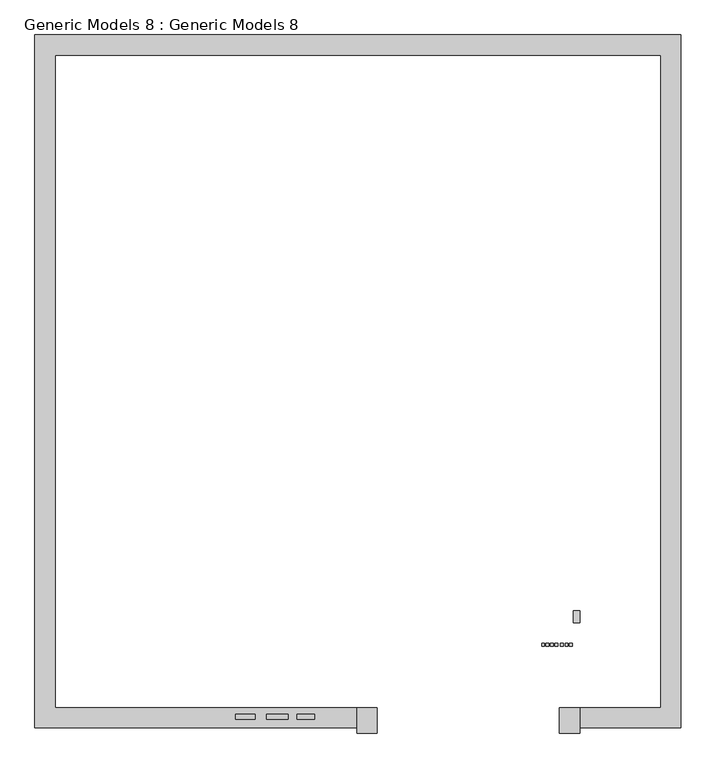
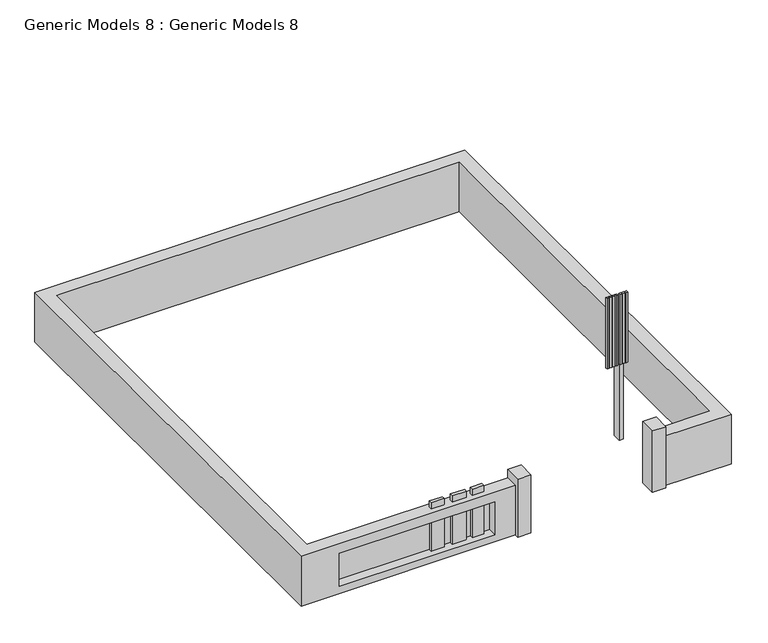
"""IFC4 building model written with IfcOpenShell, lengths in millimetres: proxy geometry, Generic Models 8 : Generic Models 8."""

from ifc_helpers import new_model, si_unit, frame, origin, origin_with_axes, place, context, project, spatial, polyline, outline, extrude, faceted_brep, source, transform, mapped, element, save


def generic_models_8_generic_models_8_408287a0(model_context):
    return source(origin(), model_context, "Body", "SolidModel", [
        extrude(outline(polyline([(-17047.091855, -16063.9538163), (-17567.791855, -16063.9538163), (-17567.791855, -15936.9538163), (-17047.091855, -15936.9538163), (-17047.091855, -16063.9538163)])), origin_with_axes(), (0.0, 0.0, 1.0), 2032.0),
        extrude(outline(polyline([(-16170.791855, -16063.9538163), (-16737.6942581, -16063.9538163), (-16737.6942581, -15936.9538163), (-16170.791855, -15936.9538163), (-16170.791855, -16063.9538163)])), origin_with_axes(), (0.0, 0.0, 1.0), 2032.0),
        extrude(outline(polyline([(-15479.5538452, -16063.9538163), (-15942.191855, -16063.9538163), (-15942.191855, -15936.9538163), (-15479.5538452, -15936.9538163), (-15479.5538452, -16063.9538163)])), origin_with_axes(), (0.0, 0.0, 1.0), 2032.0),
        faceted_brep([(-22861.0806893, -16292.5538163, -304.8), (-22861.0806893, -16292.5538163, 1774.1183755), (-22861.0806893, 1987.5639573, 1774.1183755), (-22861.0806893, 1987.5639573, -304.8), (-22327.6806893, -15759.1538163, -304.8), (-22327.6806893, 1454.1639573, -304.8), (-22327.6806893, 1454.1639573, 1774.1183755), (-22327.6806893, -15759.1538163, 1774.1183755), (-14356.9883599, -15759.1538163, 1774.1183755), (-6340.991855, 1454.1639573, 1774.1183755), (-6340.991855, -15759.1538163, 1774.1183755), (-8474.591855, -15759.1538163, 1774.1183755), (-8474.591855, -16292.5538163, 1774.1183755), (-5807.591855, -16292.5538163, 1774.1183755), (-5807.591855, 1987.5639573, 1774.1183755), (-14356.9883599, -16292.5538163, 1774.1183755), (-14356.9883599, -15759.1538163, -304.8), (-14356.9883599, -16292.5538163, -304.8), (-5807.591855, 1987.5639573, -304.8), (-5807.591855, -16292.5538163, -304.8), (-8474.591855, -16292.5538163, -304.8), (-8474.591855, -15759.1538163, -304.8), (-6340.991855, -15759.1538163, -304.8), (-6340.991855, 1454.1639573, -304.8), (-21339.6745725, -16292.5538163, 0.0), (-21339.6745725, -16292.5538163, 1367.1932574), (-15180.2427002, -16292.5538163, 1367.1932574), (-15180.2427002, -16292.5538163, 0.0), (-21339.6745725, -15936.9538163, 0.0), (-15180.2427002, -15936.9538163, 0.0), (-15180.2427002, -15936.9538163, 1367.1932574), (-21339.6745725, -15936.9538163, 1367.1932574)], [[[0, 1, 2, 3]], [[4, 5, 6, 7]], [[8, 7, 6, 9, 10, 11, 12, 13, 14, 2, 1, 15]], [[4, 16, 17, 0, 3, 18, 19, 20, 21, 22, 23, 5]], [[1, 0, 17, 15], [24, 25, 26, 27]], [[7, 8, 16, 4]], [[15, 17, 16, 8]], [[3, 2, 14, 18]], [[5, 23, 9, 6]], [[14, 13, 19, 18]], [[9, 23, 22, 10]], [[19, 13, 12, 20]], [[22, 21, 11, 10]], [[20, 12, 11, 21]], [[28, 29, 30, 31]], [[28, 31, 25, 24]], [[31, 30, 26, 25]], [[30, 29, 27, 26]], [[29, 28, 24, 27]]]),
        extrude(outline(polyline([(-9007.991855, -16432.2538163), (-9007.991855, -15759.1538163), (-8474.591855, -15759.1538163), (-8474.591855, -16432.2538163), (-9007.991855, -16432.2538163)])), frame((0.0, 0.0, -304.8), z_axis=(0.0, 0.0, 1.0), x_axis=(1.0, 0.0, 0.0)), (0.0, 0.0, 1.0), 2573.6247485),
        extrude(outline(polyline([(-13823.5883599, -15759.1538163), (-13823.5883599, -16432.2538163), (-14356.9883599, -16432.2538163), (-14356.9883599, -15759.1538163), (-13823.5883599, -15759.1538163)])), frame((0.0, 0.0, -304.8), z_axis=(0.0, 0.0, 1.0), x_axis=(1.0, 0.0, 0.0)), (0.0, 0.0, 1.0), 2425.2749439),
        extrude(outline(polyline([(-8745.0065416, -14142.2712123), (-8745.0065416, -14066.0712123), (-8668.8065416, -14066.0712123), (-8668.8065416, -14142.2712123), (-8745.0065416, -14142.2712123)])), frame((0.0, 0.0, 3657.6), z_axis=(0.0, 0.0, 1.0), x_axis=(1.0, 0.0, 0.0)), (0.0, 0.0, 1.0), 2947.4090514),
        extrude(outline(polyline([(-8860.899741, -14142.2712123), (-8860.899741, -14066.0712123), (-8789.0197051, -14066.0712123), (-8789.0197051, -14142.2712123), (-8860.899741, -14142.2712123)])), frame((0.0, 0.0, 3657.6), z_axis=(0.0, 0.0, 1.0), x_axis=(1.0, 0.0, 0.0)), (0.0, 0.0, 1.0), 2947.4090514),
        extrude(outline(polyline([(-8984.8308374, -14142.2712123), (-8984.8308374, -14066.0712123), (-8905.5149357, -14066.0712123), (-8905.5149357, -14142.2712123), (-8984.8308374, -14142.2712123)])), frame((0.0, 0.0, 3657.6), z_axis=(0.0, 0.0, 1.0), x_axis=(1.0, 0.0, 0.0)), (0.0, 0.0, 1.0), 2947.4090514),
        extrude(outline(polyline([(-9127.3515983, -14142.2712123), (-9127.3515983, -14066.0712123), (-9051.7536295, -14066.0712123), (-9051.7536295, -14142.2712123), (-9127.3515983, -14142.2712123)])), frame((0.0, 0.0, 3657.6), z_axis=(0.0, 0.0, 1.0), x_axis=(1.0, 0.0, 0.0)), (0.0, 0.0, 1.0), 2947.4090514),
        extrude(outline(polyline([(-9255.0006276, -14142.2712123), (-9255.0006276, -14066.0712123), (-9173.206104, -14066.0712123), (-9173.206104, -14142.2712123), (-9255.0006276, -14142.2712123)])), frame((0.0, 0.0, 3657.6), z_axis=(0.0, 0.0, 1.0), x_axis=(1.0, 0.0, 0.0)), (0.0, 0.0, 1.0), 2947.4090514),
        extrude(outline(polyline([(-9367.7779254, -14142.2712123), (-9367.7779254, -14066.0712123), (-9294.6585785, -14066.0712123), (-9294.6585785, -14142.2712123), (-9367.7779254, -14142.2712123)])), frame((0.0, 0.0, 3657.6), z_axis=(0.0, 0.0, 1.0), x_axis=(1.0, 0.0, 0.0)), (0.0, 0.0, 1.0), 2947.4090514),
        extrude(outline(polyline([(-9481.7945341, -14142.2712123), (-9481.7945341, -14066.0712123), (-9408.6751872, -14066.0712123), (-9408.6751872, -14142.2712123), (-9481.7945341, -14142.2712123)])), frame((0.0, 0.0, 3657.6), z_axis=(0.0, 0.0, 1.0), x_axis=(1.0, 0.0, 0.0)), (0.0, 0.0, 1.0), 2947.4090514),
        extrude(outline(polyline([(-8650.3607234, -13523.9538163), (-8650.3607234, -13199.1464347), (-8474.591855, -13199.1464347), (-8474.591855, -13523.9538163), (-8650.3607234, -13523.9538163)])), origin_with_axes(), (0.0, 0.0, 1.0), 3150.5840126),
    ])


if __name__ == "__main__":
    model = new_model("IFC4")
    model_context = context("Model", 3, world=origin())
    ifc_project = project(units=[si_unit("LENGTHUNIT", "METRE", prefix="MILLI")], contexts=[model_context])
    site = spatial("IfcSite", under=ifc_project)
    building = spatial("IfcBuilding", under=site)
    placement = place(None, origin())
    generic_models_8_generic_models_8_shape = generic_models_8_generic_models_8_408287a0(model_context)
    element("IfcBuildingElementProxy", 1, Name="Generic Models 8 : Generic Models 8", ObjectType="Generic Models 8 : Generic Models 8", at=placement, inside=building, context=model_context, shape_type="MappedRepresentation", body=[
        mapped(generic_models_8_generic_models_8_shape, transform((0.0, 0.0, 0.0), x_axis=(1.0, 0.0, 0.0), y_axis=(0.0, 1.0, 0.0), z_axis=(0.0, 0.0, 1.0))),
    ])
    save(model, "model.ifc")
